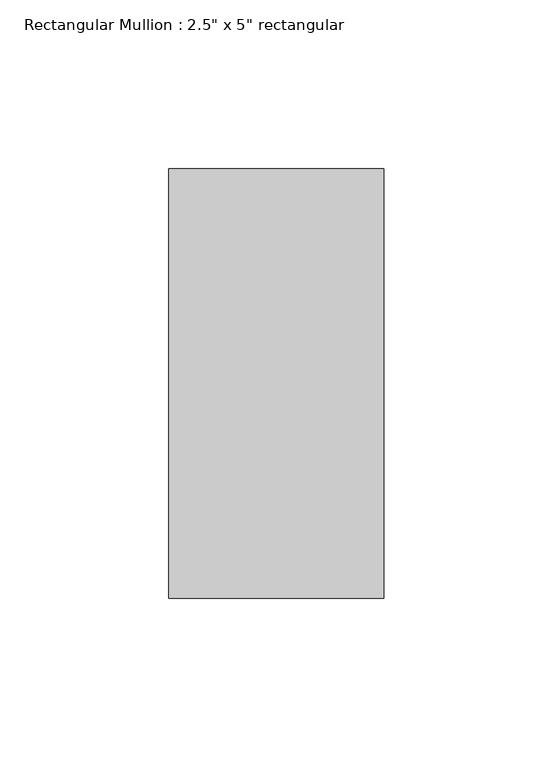
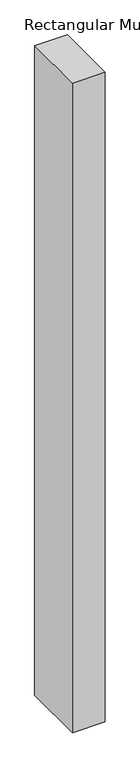
"""IFC4 building model written with IfcOpenShell, lengths in millimetres: member geometry."""

from ifc_helpers import new_model, si_unit, frame, origin, place, context, project, spatial, polyline, outline, extrude, source, transform, mapped, element, save


def member_0bf151aa(model_context):
    return source(origin(), model_context, "Body", "SweptSolid", [
        extrude(outline(polyline([(31.75, 63.5), (31.75, -63.5), (-31.75, -63.5), (-31.75, 63.5), (31.75, 63.5)])), frame((0.0, 0.0, -1335.6166668), z_axis=(0.0, 0.0, 1.0), x_axis=(1.0, 0.0, 0.0)), (0.0, 0.0, 1.0), 1335.6166668),
    ])


if __name__ == "__main__":
    model = new_model("IFC4")
    model_context = context("Model", 3, world=origin())
    ifc_project = project(units=[si_unit("LENGTHUNIT", "METRE", prefix="MILLI")], contexts=[model_context])
    site = spatial("IfcSite", under=ifc_project)
    building = spatial("IfcBuilding", under=site)
    placement = place(None, origin())
    member_shape = member_0bf151aa(model_context)
    element("IfcMember", 1, ObjectType="Rectangular Mullion : 2.5\" x 5\" rectangular", at=placement, inside=building, context=model_context, shape_type="MappedRepresentation", body=[
        mapped(member_shape, transform((0.0, 0.0, 0.0), x_axis=(1.0, 0.0, 0.0), y_axis=(0.0, 1.0, 0.0), z_axis=(0.0, 0.0, 1.0))),
    ])
    save(model, "model.ifc")

# Revit data of these elements
# Type "Rectangular Mullion : 2.5\" x 5\" rectangular"
#   built-in parameter 1007304 = 0.416667 (stored number, unit not read)
#   built-in parameter 1007301 = 0.104167 (stored number, unit not read)
#   built-in parameter 1007300 = 0.104167 (stored number, unit not read)
# Element 1 (IfcMember, "Rectangular Mullion : 2.5\" x 5\" rectangular")
#   Materials on its faces: "Aluminum"
# Materials
#   "Aluminum": class "Metal", colour RGB 247 247 247, transparency 0, Description = "Aluminum 6061", Cost = 0
